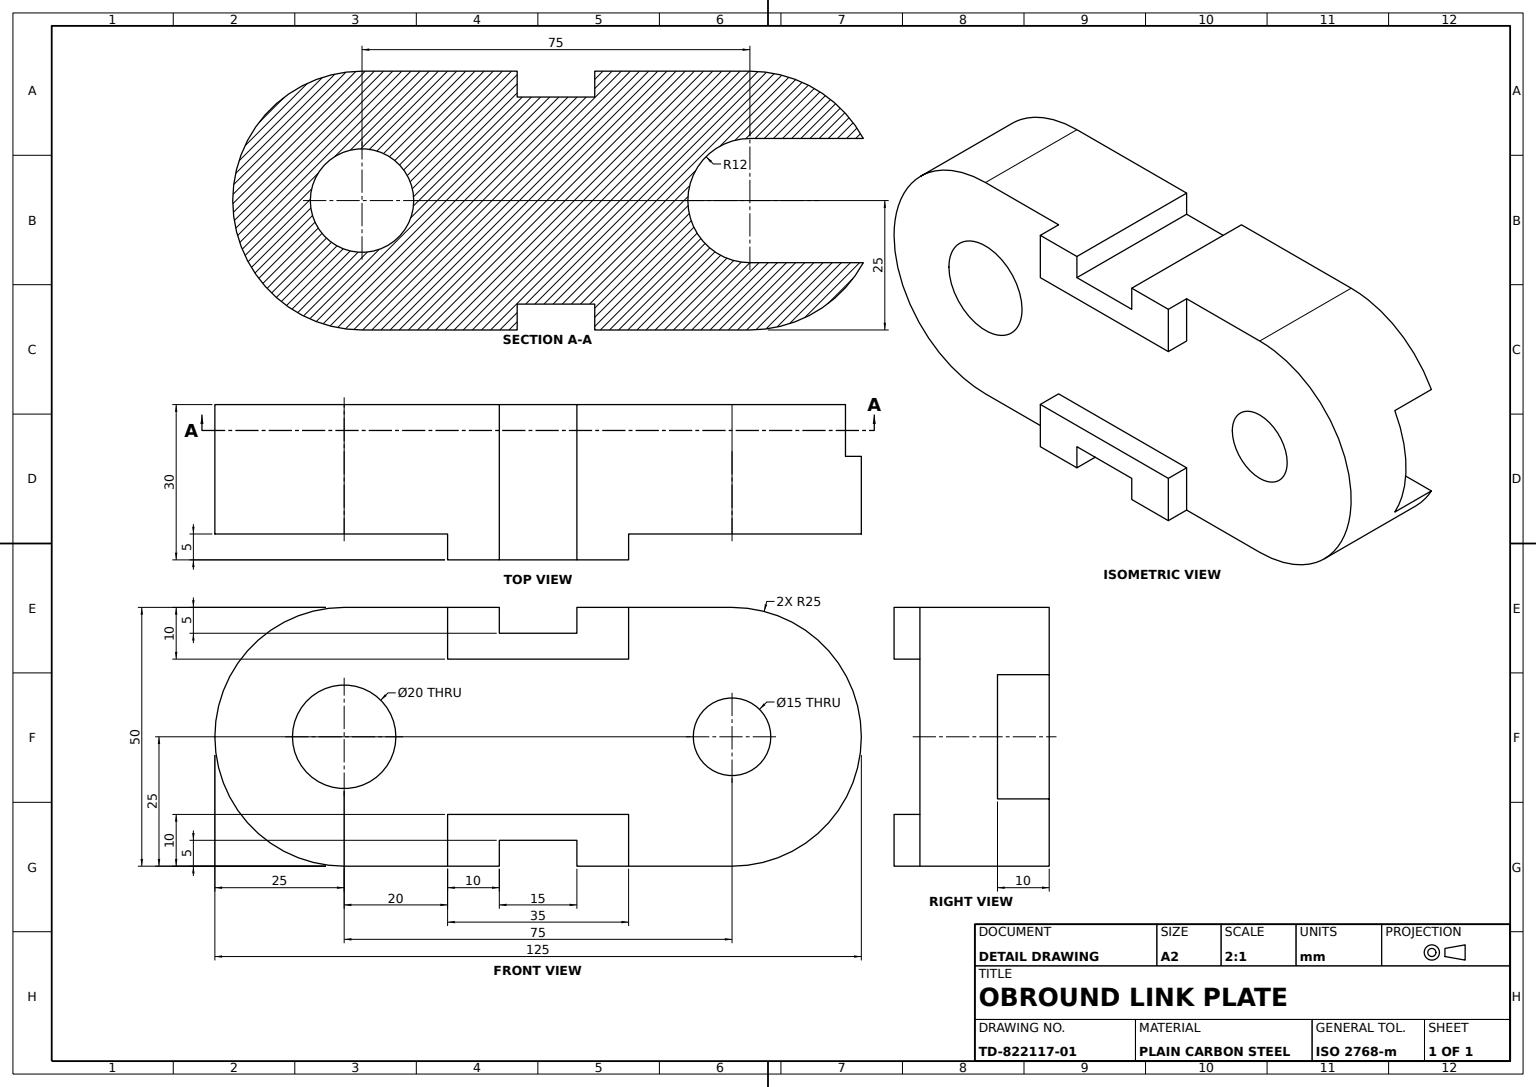
SolidWorks part; units mm, degrees
material "Plain Carbon Steel"
ref_plane "Front Plane" through (0, 0, 0) normal (0, 0, 1) x (1, 0, 0)
ref_plane "Top Plane" through (0, 0, 0) normal (0, 1, 0) x (1, 0, 0)
ref_plane "Right Plane" through (0, 0, 0) normal (1, 0, 0) x (0, 0, -1)
sketch "Link Profile Sketch" plane through (0, 0, 0) normal (0, 0, 1) x (1, 0, 0)
  line L0 (-37.5, 25) -> (37.5, 25)
  line L1 (-37.5, -25) -> (37.5, -25)
  arc A0 (37.5, -25) -> (37.5, 25) centre (37.5, 0) ccw
  arc A1 (-37.5, 25) -> (-37.5, -25) centre (-37.5, 0) ccw
  dimension "D1" = 25
  dimension "D2" = 75
  dimension "D3" = 37.5
extrude "Link Body" add sketch "Link Profile Sketch" along normal blind 25
sketch "Side Pads Sketch" plane through (0, 0, 25) normal (0, 0, 1) x (1, 0, 0)
  line L1 (-37.5, -25) -> (37.5, -25) construction
  line L2 (0, -15) -> (17.5, -15)
  line L3 (17.5, -15) -> (17.5, -25)
  line L4 (17.5, -25) -> (-17.5, -25)
  line L5 (-17.5, -25) -> (-17.5, -15)
  line L6 (-17.5, -15) -> (0, -15)
  line L7 (-17.5, 15) -> (0, 15)
  line L8 (-17.5, 25) -> (-17.5, 15)
  line L9 (17.5, 25) -> (-17.5, 25)
  line L10 (17.5, 15) -> (17.5, 25)
  line L11 (0, 15) -> (17.5, 15)
  dimension "D1" = 35
  dimension "D2" = 10
  dimension "D3" = 17.5
  dimension "D4" = 35
  dimension "D5" = 10
  dimension "D6" = 17.5
  dimension "D7" = 17.5
  dimension "D8" = 17.5
  dimension "D9" = 25
extrude "Side Pads 35x10" add sketch "Side Pads Sketch" along normal blind 5
sketch "T-Slots Sketch" plane through (0, 0, 30) normal (0, 0, 1) x (1, 0, 0)
  line L2 (0, -20) -> (7.5, -20)
  line L3 (7.5, -20) -> (7.5, -26.5387)
  line L4 (7.5, -26.5387) -> (-7.5, -26.5387)
  line L5 (-7.5, -26.5387) -> (-7.5, -20)
  line L6 (-7.5, -20) -> (0, -20)
  line L7 (-7.5, 20) -> (0, 20)
  line L8 (-7.5, 26.5387) -> (-7.5, 20)
  line L9 (7.5, 26.5387) -> (-7.5, 26.5387)
  line L10 (7.5, 20) -> (7.5, 26.5387)
  line L11 (0, 20) -> (7.5, 20)
  dimension "D1" = 15
  dimension "D2" = 6.5387
  dimension "D3" = 26.5387
  dimension "D4" = 7.5
  dimension "D5" = 15
  dimension "D6" = 6.5387
  dimension "D7" = 26.5387
  dimension "D8" = 7.5
  dimension "D9" = 7.5
extrude "T-Slots" cut sketch "T-Slots Sketch" against normal blind 35
sketch "Cross Slot Sketch" plane through (0, 0, 0) normal (0, 0, -1) x (-1, 0, 0)
  line L0 (-37.5, 12) -> (-67.446, 12)
  line L1 (-37.5, -12) -> (-67.446, -12)
  line L2 (-67.446, -12) -> (-67.446, 12)
  arc A0 (-37.5, -12) -> (-37.5, 12) centre (-37.5, 0) ccw
  dimension "D1" = 12
  dimension "D2" = 67.446
extrude "Cross Slot 12mm" cut sketch "Cross Slot Sketch" against normal blind 10
sketch "Eye Bore Ø20 Sketch" plane through (0, 0, 25) normal (0, 0, 1) x (1, 0, 0)
  circle A0 centre (-37.5, 0) radius 10
  dimension "D1" = 20
extrude "Eye Bore Ø20" cut sketch "Eye Bore Ø20 Sketch" against normal blind 32
sketch "Eye Bore Ø15 Sketch" plane through (0, 0, 25) normal (0, 0, 1) x (1, 0, 0)
  circle A0 centre (37.5, 0) radius 7.5
  dimension "D1" = 15
extrude "Eye Bore Ø15" cut sketch "Eye Bore Ø15 Sketch" against normal blind 32
